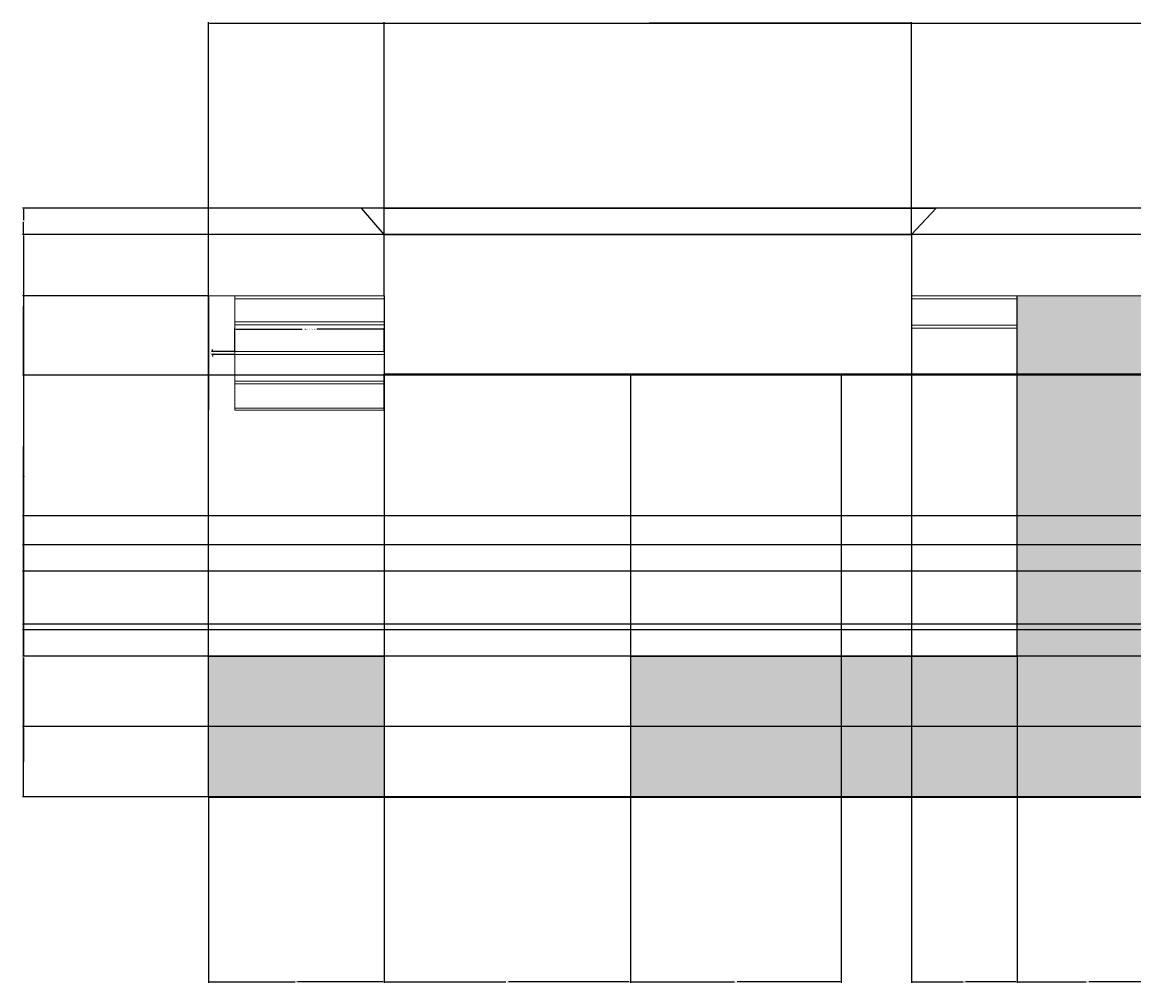
# Model space of a CAD drawing. Units: inches. Extents: x 2121 to 2815, y 1818 to 2233.
# Tile 1 of 6: x 2121 to 2311, y 1818 to 1982. Entities that reach past the tile are written whole.
import ezdxf

# ---------------------------------------------------------------- set-up
doc = ezdxf.new("R2010")
doc.units = ezdxf.units.IN
for name, color, linetype, lineweight in [('A-ANNO-DIMS', 2, 'Continuous', 18), ('A-ELEV', 7, 'Continuous', 25), ('A-ELEV-GRDE', 7, 'Continuous', 35), ('A-ELEV-SLAT', 7, 'Continuous', 18), ('A-WALL-COPG', 7, 'Continuous', 25), ('A-WALL-PATT', 8, 'Continuous', 13)]:
    doc.layers.add(name, color=color, linetype=linetype, lineweight=lineweight)
doc.styles.get("Standard").update_dxf_attribs({"font": 'arial.ttf'})
doc.dimstyles.get("Standard").update_dxf_attribs({"dimtxt": 0.18, "dimasz": 0.18, "dimexe": 0.18, "dimexo": 0.0625, "dimgap": 0.09, "dimtad": 0, "dimtih": 1, "dimtoh": 1, "dimdec": 4, "dimzin": 0, "dimdsep": 46, "dimtxsty": 'Standard', "dimcen": 0.09, "dimadec": 0, "dimazin": 0, "dimtfac": 1, "dimtdec": 4, "dimtofl": 0, "dimtmove": 0, "dimatfit": 3, "dimfxl": 1, "dimtolj": 1, "dimtzin": 0, "dimarcsym": 0})

# ---------------------------------------------------------------- blocks, each defined once
blk = doc.blocks.new('WALL-SLAT-25_5')
for p, q in [((0, 0.5), (25.5, 0.5)), ((0, 0), (25.5, 0))]:
    blk.add_line(p, q)
blk = doc.blocks.new('*D8')
at = {"layer": 'A-ANNO-DIMS', "color": 0, "lineweight": -2, "transparency": 16777216}
for p, q in [((2157.33, 1925.97), (2157.33, 1929.92)), ((2157.51, 1929.74), (2168.82, 1929.74)), ((2182.65, 1929.74), (2171.35, 1929.74)), ((2182.83, 1925.97), (2182.83, 1929.92))]:
    blk.add_line(p, q, dxfattribs=at)
at = {"layer": 'A-ANNO-DIMS', "color": 0, "transparency": 16777216}
for points in [[(2157.51, 1929.77), (2157.51, 1929.71), (2157.33, 1929.74)], [(2182.65, 1929.77), (2182.65, 1929.71), (2182.83, 1929.74)]]:
    blk.add_solid(points, dxfattribs=at)
at = {"layer": 'Defpoints', "color": 0, "transparency": 16777216}
for p in [(2182.83, 1929.74), (2157.33, 1925.91), (2182.83, 1925.91)]:
    blk.add_point(p, dxfattribs=at)
at = {"layer": 'A-ANNO-DIMS', "color": 0, "transparency": 16777216, "insert": (2170.08, 1929.74), "char_height": 0.18, "attachment_point": 5}
blk.add_mtext('\\A1;LONG SLAT 26 TYP.', dxfattribs=at)
blk = doc.blocks.new('*D9')
at = {"layer": 'A-ANNO-DIMS', "color": 0, "lineweight": -2, "transparency": 16777216}
for p, q in [((2157.27, 1925.91), (2153.33, 1925.91)), ((2157.27, 1925.41), (2153.33, 1925.41)), ((2153.51, 1926.09), (2153.51, 1926.27)), ((2153.51, 1925.23), (2153.51, 1925.05))]:
    blk.add_line(p, q, dxfattribs=at)
at = {"layer": 'A-ANNO-DIMS', "color": 0, "transparency": 16777216}
for points in [[(2153.48, 1926.09), (2153.54, 1926.09), (2153.51, 1925.91)], [(2153.48, 1925.23), (2153.54, 1925.23), (2153.51, 1925.41)]]:
    blk.add_solid(points, dxfattribs=at)
at = {"layer": 'Defpoints', "color": 0, "transparency": 16777216}
for p in [(2153.51, 1925.91), (2157.33, 1925.91), (2157.33, 1925.41)]:
    blk.add_point(p, dxfattribs=at)
at = {"layer": 'A-ANNO-DIMS', "color": 0, "transparency": 16777216, "insert": (2153.51, 1925.66), "char_height": 0.18, "attachment_point": 5}
blk.add_mtext('\\A1;1 TYP.', dxfattribs=at)
blk = doc.blocks.new('*D43')
at = {"layer": 'A-ANNO-DIMS', "color": 0, "lineweight": -2, "transparency": 16777216}
for p, q in [((2152.83, 1935.47), (2152.83, 1982.13)), ((2153.01, 1981.95), (2398.33, 1981.95)), ((2644.45, 1981.95), (2399.13, 1981.95)), ((2644.63, 1950.47), (2644.63, 1982.13))]:
    blk.add_line(p, q, dxfattribs=at)
at = {"layer": 'A-ANNO-DIMS', "color": 0, "transparency": 16777216}
for points in [[(2153.01, 1981.98), (2153.01, 1981.92), (2152.83, 1981.95)], [(2644.45, 1981.98), (2644.45, 1981.92), (2644.63, 1981.95)]]:
    blk.add_solid(points, dxfattribs=at)
at = {"layer": 'Defpoints', "color": 0, "transparency": 16777216}
for p in [(2644.63, 1981.95), (2644.63, 1950.41), (2152.83, 1935.41)]:
    blk.add_point(p, dxfattribs=at)
at = {"layer": 'A-ANNO-DIMS', "color": 0, "transparency": 16777216, "insert": (2398.73, 1981.95), "char_height": 0.18, "attachment_point": 5}
blk.add_mtext('\\A1;491.8', dxfattribs=at)
blk = doc.blocks.new('*D45')
at = {"layer": 'A-ANNO-DIMS', "color": 0, "lineweight": -2, "transparency": 16777216}
for p, q in [((2152.77, 1873.91), (2121.11, 1873.91)), ((2121.29, 1873.73), (2121.29, 1862.09)), ((2121.29, 1850.09), (2121.29, 1861.73)), ((2152.77, 1849.91), (2121.11, 1849.91))]:
    blk.add_line(p, q, dxfattribs=at)
at = {"layer": 'A-ANNO-DIMS', "color": 0, "transparency": 16777216}
for points in [[(2121.26, 1873.73), (2121.32, 1873.73), (2121.29, 1873.91)], [(2121.26, 1850.09), (2121.32, 1850.09), (2121.29, 1849.91)]]:
    blk.add_solid(points, dxfattribs=at)
at = {"layer": 'Defpoints', "color": 0, "transparency": 16777216}
for p in [(2121.29, 1873.91), (2152.83, 1873.91), (2152.83, 1849.91)]:
    blk.add_point(p, dxfattribs=at)
at = {"layer": 'A-ANNO-DIMS', "color": 0, "transparency": 16777216, "insert": (2121.29, 1861.91), "char_height": 0.18, "attachment_point": 5}
blk.add_mtext('\\A1;24', dxfattribs=at)
blk = doc.blocks.new('*D46')
at = {"layer": 'A-ANNO-DIMS', "color": 0, "lineweight": -2, "transparency": 16777216}
for p, q in [((2152.77, 1935.41), (2121.11, 1935.41)), ((2121.29, 1935.23), (2121.29, 1904.84)), ((2121.29, 1874.09), (2121.29, 1904.48)), ((2152.77, 1873.91), (2121.11, 1873.91))]:
    blk.add_line(p, q, dxfattribs=at)
at = {"layer": 'A-ANNO-DIMS', "color": 0, "transparency": 16777216}
for points in [[(2121.26, 1935.23), (2121.32, 1935.23), (2121.29, 1935.41)], [(2121.26, 1874.09), (2121.32, 1874.09), (2121.29, 1873.91)]]:
    blk.add_solid(points, dxfattribs=at)
at = {"layer": 'Defpoints', "color": 0, "transparency": 16777216}
for p in [(2121.29, 1935.41), (2152.83, 1935.41), (2152.83, 1873.91)]:
    blk.add_point(p, dxfattribs=at)
at = {"layer": 'A-ANNO-DIMS', "color": 0, "transparency": 16777216, "insert": (2121.29, 1904.66), "char_height": 0.18, "attachment_point": 5}
blk.add_mtext('\\A1;61.5', dxfattribs=at)
blk = doc.blocks.new('*D47')
at = {"layer": 'A-ANNO-DIMS', "color": 0, "lineweight": -2, "transparency": 16777216}
for p, q in [((2152.83, 1849.84), (2152.83, 1818.19)), ((2182.83, 1849.84), (2182.83, 1818.19)), ((2153.01, 1818.37), (2167.61, 1818.37)), ((2182.65, 1818.37), (2168.05, 1818.37))]:
    blk.add_line(p, q, dxfattribs=at)
at = {"layer": 'A-ANNO-DIMS', "color": 0, "transparency": 16777216}
for points in [[(2153.01, 1818.4), (2153.01, 1818.34), (2152.83, 1818.37)], [(2182.65, 1818.4), (2182.65, 1818.34), (2182.83, 1818.37)]]:
    blk.add_solid(points, dxfattribs=at)
at = {"layer": 'Defpoints', "color": 0, "transparency": 16777216}
for p in [(2152.83, 1849.91), (2182.83, 1849.91), (2182.83, 1818.37)]:
    blk.add_point(p, dxfattribs=at)
at = {"layer": 'A-ANNO-DIMS', "color": 0, "transparency": 16777216, "insert": (2167.83, 1818.37), "char_height": 0.18, "attachment_point": 5}
blk.add_mtext('\\A1;30', dxfattribs=at)
blk = doc.blocks.new('*D48')
at = {"layer": 'A-ANNO-DIMS', "color": 0, "lineweight": -2, "transparency": 16777216}
for p, q in [((2182.83, 1849.84), (2182.83, 1818.19)), ((2224.83, 1849.84), (2224.83, 1818.19)), ((2183.01, 1818.37), (2203.61, 1818.37)), ((2224.65, 1818.37), (2204.05, 1818.37))]:
    blk.add_line(p, q, dxfattribs=at)
at = {"layer": 'A-ANNO-DIMS', "color": 0, "transparency": 16777216}
for points in [[(2183.01, 1818.4), (2183.01, 1818.34), (2182.83, 1818.37)], [(2224.65, 1818.4), (2224.65, 1818.34), (2224.83, 1818.37)]]:
    blk.add_solid(points, dxfattribs=at)
at = {"layer": 'Defpoints', "color": 0, "transparency": 16777216}
for p in [(2182.83, 1849.91), (2224.83, 1849.91), (2224.83, 1818.37)]:
    blk.add_point(p, dxfattribs=at)
at = {"layer": 'A-ANNO-DIMS', "color": 0, "transparency": 16777216, "insert": (2203.83, 1818.37), "char_height": 0.18, "attachment_point": 5}
blk.add_mtext('\\A1;42', dxfattribs=at)
blk = doc.blocks.new('*D49')
at = {"layer": 'A-ANNO-DIMS', "color": 0, "lineweight": -2, "transparency": 16777216}
for p, q in [((2182.83, 1945.97), (2182.83, 1982.13)), ((2183.01, 1981.95), (2227.61, 1981.95)), ((2272.65, 1981.95), (2228.05, 1981.95)), ((2272.83, 1945.97), (2272.83, 1982.13))]:
    blk.add_line(p, q, dxfattribs=at)
at = {"layer": 'A-ANNO-DIMS', "color": 0, "transparency": 16777216}
for points in [[(2183.01, 1981.98), (2183.01, 1981.92), (2182.83, 1981.95)], [(2272.65, 1981.98), (2272.65, 1981.92), (2272.83, 1981.95)]]:
    blk.add_solid(points, dxfattribs=at)
at = {"layer": 'Defpoints', "color": 0, "transparency": 16777216}
for p in [(2272.83, 1981.95), (2182.83, 1945.91), (2272.83, 1945.91)]:
    blk.add_point(p, dxfattribs=at)
at = {"layer": 'A-ANNO-DIMS', "color": 0, "transparency": 16777216, "insert": (2227.83, 1981.95), "char_height": 0.18, "attachment_point": 5}
blk.add_mtext('\\A1;90', dxfattribs=at)
blk = doc.blocks.new('*D50')
at = {"layer": 'A-ANNO-DIMS', "color": 0, "lineweight": -2, "transparency": 16777216}
for p, q in [((2272.83, 1873.84), (2272.83, 1818.19)), ((2290.83, 1873.84), (2290.83, 1818.19)), ((2273.01, 1818.37), (2281.62, 1818.37)), ((2290.65, 1818.37), (2282.04, 1818.37))]:
    blk.add_line(p, q, dxfattribs=at)
at = {"layer": 'A-ANNO-DIMS', "color": 0, "transparency": 16777216}
for points in [[(2273.01, 1818.4), (2273.01, 1818.34), (2272.83, 1818.37)], [(2290.65, 1818.4), (2290.65, 1818.34), (2290.83, 1818.37)]]:
    blk.add_solid(points, dxfattribs=at)
at = {"layer": 'Defpoints', "color": 0, "transparency": 16777216}
for p in [(2272.83, 1873.91), (2290.83, 1873.91), (2290.83, 1818.37)]:
    blk.add_point(p, dxfattribs=at)
at = {"layer": 'A-ANNO-DIMS', "color": 0, "transparency": 16777216, "insert": (2281.83, 1818.37), "char_height": 0.18, "attachment_point": 5}
blk.add_mtext('\\A1;18', dxfattribs=at)
blk = doc.blocks.new('*D51')
at = {"layer": 'A-ANNO-DIMS', "color": 0, "lineweight": -2, "transparency": 16777216}
for p, q in [((2290.83, 1873.84), (2290.83, 1818.19)), ((2314.83, 1873.84), (2314.83, 1818.19)), ((2291.01, 1818.37), (2302.61, 1818.37)), ((2314.65, 1818.37), (2303.05, 1818.37))]:
    blk.add_line(p, q, dxfattribs=at)
at = {"layer": 'A-ANNO-DIMS', "color": 0, "transparency": 16777216}
for points in [[(2291.01, 1818.4), (2291.01, 1818.34), (2290.83, 1818.37)], [(2314.65, 1818.4), (2314.65, 1818.34), (2314.83, 1818.37)]]:
    blk.add_solid(points, dxfattribs=at)
at = {"layer": 'Defpoints', "color": 0, "transparency": 16777216}
for p in [(2290.83, 1873.91), (2314.83, 1873.91), (2314.83, 1818.37)]:
    blk.add_point(p, dxfattribs=at)
at = {"layer": 'A-ANNO-DIMS', "color": 0, "transparency": 16777216, "insert": (2302.83, 1818.37), "char_height": 0.18, "attachment_point": 5}
blk.add_mtext('\\A1;24', dxfattribs=at)
blk = doc.blocks.new('*D59')
at = {"layer": 'A-ANNO-DIMS', "color": 0, "lineweight": -2, "transparency": 16777216}
for p, q in [((2182.9, 1922.1), (2815, 1922.1)), ((2814.82, 1921.92), (2814.82, 1886.18)), ((2814.82, 1850.09), (2814.82, 1885.82)), ((2182.9, 1849.91), (2815, 1849.91))]:
    blk.add_line(p, q, dxfattribs=at)
at = {"layer": 'A-ANNO-DIMS', "color": 0, "transparency": 16777216}
for points in [[(2814.79, 1921.92), (2814.85, 1921.92), (2814.82, 1922.1)], [(2814.79, 1850.09), (2814.85, 1850.09), (2814.82, 1849.91)]]:
    blk.add_solid(points, dxfattribs=at)
at = {"layer": 'Defpoints', "color": 0, "transparency": 16777216}
for p in [(2182.83, 1922.1), (2814.82, 1922.1), (2182.83, 1849.91)]:
    blk.add_point(p, dxfattribs=at)
at = {"layer": 'A-ANNO-DIMS', "color": 0, "transparency": 16777216, "insert": (2814.82, 1886), "char_height": 0.18, "attachment_point": 5}
blk.add_mtext('\\A1;72.2', dxfattribs=at)
blk = doc.blocks.new('*D60')
at = {"layer": 'A-ANNO-DIMS', "color": 0, "lineweight": -2, "transparency": 16777216}
for p, q in [((2224.83, 1873.84), (2224.83, 1818.19)), ((2260.83, 1873.84), (2260.83, 1818.19)), ((2225.01, 1818.37), (2242.61, 1818.37)), ((2260.65, 1818.37), (2243.05, 1818.37))]:
    blk.add_line(p, q, dxfattribs=at)
at = {"layer": 'A-ANNO-DIMS', "color": 0, "transparency": 16777216}
for points in [[(2225.01, 1818.4), (2225.01, 1818.34), (2224.83, 1818.37)], [(2260.65, 1818.4), (2260.65, 1818.34), (2260.83, 1818.37)]]:
    blk.add_solid(points, dxfattribs=at)
at = {"layer": 'Defpoints', "color": 0, "transparency": 16777216}
for p in [(2224.83, 1873.91), (2260.83, 1873.91), (2260.83, 1818.37)]:
    blk.add_point(p, dxfattribs=at)
at = {"layer": 'A-ANNO-DIMS', "color": 0, "transparency": 16777216, "insert": (2242.83, 1818.37), "char_height": 0.18, "attachment_point": 5}
blk.add_mtext('\\A1;36', dxfattribs=at)
blk = doc.blocks.new('*D61')
at = {"layer": 'A-ANNO-DIMS', "color": 0, "lineweight": -2, "transparency": 16777216}
for p, q in [((2314.77, 1861.91), (2121.11, 1861.91)), ((2121.29, 1861.73), (2121.29, 1856.09)), ((2121.29, 1850.09), (2121.29, 1855.73)), ((2314.77, 1849.91), (2121.11, 1849.91))]:
    blk.add_line(p, q, dxfattribs=at)
at = {"layer": 'A-ANNO-DIMS', "color": 0, "transparency": 16777216}
for points in [[(2121.26, 1861.73), (2121.32, 1861.73), (2121.29, 1861.91)], [(2121.26, 1850.09), (2121.32, 1850.09), (2121.29, 1849.91)]]:
    blk.add_solid(points, dxfattribs=at)
at = {"layer": 'Defpoints', "color": 0, "transparency": 16777216}
for p in [(2121.29, 1861.91), (2314.83, 1861.91), (2314.83, 1849.91)]:
    blk.add_point(p, dxfattribs=at)
at = {"layer": 'A-ANNO-DIMS', "color": 0, "transparency": 16777216, "insert": (2121.29, 1855.91), "char_height": 0.18, "attachment_point": 5}
blk.add_mtext('\\A1;12', dxfattribs=at)
blk = doc.blocks.new('*D63')
at = {"layer": 'A-ANNO-DIMS', "color": 0, "lineweight": -2, "transparency": 16777216}
for p, q in [((2347.77, 1892.91), (2121.11, 1892.91)), ((2121.29, 1892.73), (2121.29, 1890.84)), ((2121.29, 1888.59), (2121.29, 1890.48)), ((2347.77, 1888.41), (2121.11, 1888.41))]:
    blk.add_line(p, q, dxfattribs=at)
at = {"layer": 'A-ANNO-DIMS', "color": 0, "transparency": 16777216}
for points in [[(2121.26, 1892.73), (2121.32, 1892.73), (2121.29, 1892.91)], [(2121.26, 1888.59), (2121.32, 1888.59), (2121.29, 1888.41)]]:
    blk.add_solid(points, dxfattribs=at)
at = {"layer": 'Defpoints', "color": 0, "transparency": 16777216}
for p in [(2121.29, 1892.91), (2347.83, 1892.91), (2347.83, 1888.41)]:
    blk.add_point(p, dxfattribs=at)
at = {"layer": 'A-ANNO-DIMS', "color": 0, "transparency": 16777216, "insert": (2121.29, 1890.66), "char_height": 0.18, "attachment_point": 5}
blk.add_mtext('\\A1;4.5', dxfattribs=at)
blk = doc.blocks.new('*D64')
at = {"layer": 'A-ANNO-DIMS', "color": 0, "lineweight": -2, "transparency": 16777216}
for p, q in [((2347.77, 1879.41), (2121.11, 1879.41)), ((2121.29, 1879.23), (2121.29, 1876.84)), ((2121.29, 1874.09), (2121.29, 1876.48)), ((2314.77, 1873.91), (2121.11, 1873.91))]:
    blk.add_line(p, q, dxfattribs=at)
at = {"layer": 'A-ANNO-DIMS', "color": 0, "transparency": 16777216}
for points in [[(2121.26, 1879.23), (2121.32, 1879.23), (2121.29, 1879.41)], [(2121.26, 1874.09), (2121.32, 1874.09), (2121.29, 1873.91)]]:
    blk.add_solid(points, dxfattribs=at)
at = {"layer": 'Defpoints', "color": 0, "transparency": 16777216}
for p in [(2121.29, 1879.41), (2347.83, 1879.41), (2314.83, 1873.91)]:
    blk.add_point(p, dxfattribs=at)
at = {"layer": 'A-ANNO-DIMS', "color": 0, "transparency": 16777216, "insert": (2121.29, 1876.66), "char_height": 0.18, "attachment_point": 5}
blk.add_mtext('\\A1;5.5', dxfattribs=at)
blk = doc.blocks.new('*D65')
at = {"layer": 'A-ANNO-DIMS', "color": 0, "lineweight": -2, "transparency": 16777216}
for p, q in [((2619.77, 1897.91), (2121.11, 1897.91)), ((2121.29, 1897.73), (2121.29, 1874.09)), ((2121.29, 1850.09), (2121.29, 1873.73)), ((2619.77, 1849.91), (2121.11, 1849.91))]:
    blk.add_line(p, q, dxfattribs=at)
at = {"layer": 'A-ANNO-DIMS', "color": 0, "transparency": 16777216}
for points in [[(2121.26, 1897.73), (2121.32, 1897.73), (2121.29, 1897.91)], [(2121.26, 1850.09), (2121.32, 1850.09), (2121.29, 1849.91)]]:
    blk.add_solid(points, dxfattribs=at)
at = {"layer": 'Defpoints', "color": 0, "transparency": 16777216}
for p in [(2121.29, 1897.91), (2619.83, 1897.91), (2619.83, 1849.91)]:
    blk.add_point(p, dxfattribs=at)
at = {"layer": 'A-ANNO-DIMS', "color": 0, "transparency": 16777216, "insert": (2121.29, 1873.91), "char_height": 0.18, "attachment_point": 5}
blk.add_mtext('\\A1;48', dxfattribs=at)
blk = doc.blocks.new('*D66')
at = {"layer": 'A-ANNO-DIMS', "color": 0, "lineweight": -2, "transparency": 16777216}
for p, q in [((2619.77, 1921.91), (2121.11, 1921.91)), ((2121.29, 1921.73), (2121.29, 1910.09)), ((2121.29, 1898.09), (2121.29, 1909.73)), ((2619.77, 1897.91), (2121.11, 1897.91))]:
    blk.add_line(p, q, dxfattribs=at)
at = {"layer": 'A-ANNO-DIMS', "color": 0, "transparency": 16777216}
for points in [[(2121.26, 1921.73), (2121.32, 1921.73), (2121.29, 1921.91)], [(2121.26, 1898.09), (2121.32, 1898.09), (2121.29, 1897.91)]]:
    blk.add_solid(points, dxfattribs=at)
at = {"layer": 'Defpoints', "color": 0, "transparency": 16777216}
for p in [(2121.29, 1921.91), (2619.83, 1921.91), (2619.83, 1897.91)]:
    blk.add_point(p, dxfattribs=at)
at = {"layer": 'A-ANNO-DIMS', "color": 0, "transparency": 16777216, "insert": (2121.29, 1909.91), "char_height": 0.18, "attachment_point": 5}
blk.add_mtext('\\A1;24', dxfattribs=at)
blk = doc.blocks.new('*D72')
at = {"layer": 'A-ANNO-DIMS', "color": 0, "lineweight": -2, "transparency": 16777216}
for p, q in [((2760.77, 1861.91), (2121.11, 1861.91)), ((2121.29, 1861.73), (2121.29, 1856.09)), ((2121.29, 1850.09), (2121.29, 1855.73)), ((2760.77, 1849.91), (2121.11, 1849.91))]:
    blk.add_line(p, q, dxfattribs=at)
at = {"layer": 'A-ANNO-DIMS', "color": 0, "transparency": 16777216}
for points in [[(2121.26, 1861.73), (2121.32, 1861.73), (2121.29, 1861.91)], [(2121.26, 1850.09), (2121.32, 1850.09), (2121.29, 1849.91)]]:
    blk.add_solid(points, dxfattribs=at)
at = {"layer": 'Defpoints', "color": 0, "transparency": 16777216}
for p in [(2121.29, 1861.91), (2760.83, 1861.91), (2760.83, 1849.91)]:
    blk.add_point(p, dxfattribs=at)
at = {"layer": 'A-ANNO-DIMS', "color": 0, "transparency": 16777216, "insert": (2121.29, 1855.91), "char_height": 0.18, "attachment_point": 5}
blk.add_mtext('\\A1;12', dxfattribs=at)
blk = doc.blocks.new('*D73')
at = {"layer": 'A-ANNO-DIMS', "color": 0, "lineweight": -2, "transparency": 16777216}
for p, q in [((2765.27, 1873.91), (2121.11, 1873.91)), ((2121.29, 1873.73), (2121.29, 1868.09)), ((2121.29, 1862.09), (2121.29, 1867.73)), ((2760.77, 1861.91), (2121.11, 1861.91))]:
    blk.add_line(p, q, dxfattribs=at)
at = {"layer": 'A-ANNO-DIMS', "color": 0, "transparency": 16777216}
for points in [[(2121.26, 1873.73), (2121.32, 1873.73), (2121.29, 1873.91)], [(2121.26, 1862.09), (2121.32, 1862.09), (2121.29, 1861.91)]]:
    blk.add_solid(points, dxfattribs=at)
at = {"layer": 'Defpoints', "color": 0, "transparency": 16777216}
for p in [(2121.29, 1873.91), (2765.33, 1873.91), (2760.83, 1861.91)]:
    blk.add_point(p, dxfattribs=at)
at = {"layer": 'A-ANNO-DIMS', "color": 0, "transparency": 16777216, "insert": (2121.29, 1867.91), "char_height": 0.18, "attachment_point": 5}
blk.add_mtext('\\A1;12', dxfattribs=at)
blk = doc.blocks.new('*D74')
at = {"layer": 'A-ANNO-DIMS', "color": 0, "lineweight": -2, "transparency": 16777216}
for p, q in [((2765.27, 1921.91), (2121.11, 1921.91)), ((2121.29, 1921.73), (2121.29, 1898.09)), ((2121.29, 1874.09), (2121.29, 1897.73)), ((2765.27, 1873.91), (2121.11, 1873.91))]:
    blk.add_line(p, q, dxfattribs=at)
at = {"layer": 'A-ANNO-DIMS', "color": 0, "transparency": 16777216}
for points in [[(2121.26, 1921.73), (2121.32, 1921.73), (2121.29, 1921.91)], [(2121.26, 1874.09), (2121.32, 1874.09), (2121.29, 1873.91)]]:
    blk.add_solid(points, dxfattribs=at)
at = {"layer": 'Defpoints', "color": 0, "transparency": 16777216}
for p in [(2121.29, 1921.91), (2765.33, 1921.91), (2765.33, 1873.91)]:
    blk.add_point(p, dxfattribs=at)
at = {"layer": 'A-ANNO-DIMS', "color": 0, "transparency": 16777216, "insert": (2121.29, 1897.91), "char_height": 0.18, "attachment_point": 5}
blk.add_mtext('\\A1;48', dxfattribs=at)
blk = doc.blocks.new('*D75')
at = {"layer": 'A-ANNO-DIMS', "color": 0, "lineweight": -2, "transparency": 16777216}
for p, q in [((2760.77, 1945.91), (2121.11, 1945.91)), ((2121.29, 1945.73), (2121.29, 1934.09)), ((2121.29, 1922.09), (2121.29, 1933.73)), ((2760.77, 1921.91), (2121.11, 1921.91))]:
    blk.add_line(p, q, dxfattribs=at)
at = {"layer": 'A-ANNO-DIMS', "color": 0, "transparency": 16777216}
for points in [[(2121.26, 1945.73), (2121.32, 1945.73), (2121.29, 1945.91)], [(2121.26, 1922.09), (2121.32, 1922.09), (2121.29, 1921.91)]]:
    blk.add_solid(points, dxfattribs=at)
at = {"layer": 'Defpoints', "color": 0, "transparency": 16777216}
for p in [(2121.29, 1945.91), (2760.83, 1945.91), (2760.83, 1921.91)]:
    blk.add_point(p, dxfattribs=at)
at = {"layer": 'A-ANNO-DIMS', "color": 0, "transparency": 16777216, "insert": (2121.29, 1933.91), "char_height": 0.18, "attachment_point": 5}
blk.add_mtext('\\A1;24', dxfattribs=at)
blk = doc.blocks.new('*D76')
at = {"layer": 'A-ANNO-DIMS', "color": 0, "lineweight": -2, "transparency": 16777216}
for p, q in [((2756.87, 1950.41), (2121.11, 1950.41)), ((2121.29, 1950.23), (2121.29, 1948.34)), ((2121.29, 1946.09), (2121.29, 1947.98)), ((2760.77, 1945.91), (2121.11, 1945.91))]:
    blk.add_line(p, q, dxfattribs=at)
at = {"layer": 'A-ANNO-DIMS', "color": 0, "transparency": 16777216}
for points in [[(2121.26, 1950.23), (2121.32, 1950.23), (2121.29, 1950.41)], [(2121.26, 1946.09), (2121.32, 1946.09), (2121.29, 1945.91)]]:
    blk.add_solid(points, dxfattribs=at)
at = {"layer": 'Defpoints', "color": 0, "transparency": 16777216}
for p in [(2121.29, 1950.41), (2756.93, 1950.41), (2760.83, 1945.91)]:
    blk.add_point(p, dxfattribs=at)
at = {"layer": 'A-ANNO-DIMS', "color": 0, "transparency": 16777216, "insert": (2121.29, 1948.16), "char_height": 0.18, "attachment_point": 5}
blk.add_mtext('\\A1;4.5', dxfattribs=at)
blk = doc.blocks.new('*D82')
at = {"layer": 'A-ANNO-DIMS', "color": 0, "lineweight": -2, "transparency": 16777216}
for p, q in [((2769.77, 1878.41), (2121.11, 1878.41)), ((2121.29, 1878.23), (2121.29, 1876.34)), ((2121.29, 1874.09), (2121.29, 1875.98)), ((2769.77, 1873.91), (2121.11, 1873.91))]:
    blk.add_line(p, q, dxfattribs=at)
at = {"layer": 'A-ANNO-DIMS', "color": 0, "transparency": 16777216}
for points in [[(2121.26, 1878.23), (2121.32, 1878.23), (2121.29, 1878.41)], [(2121.26, 1874.09), (2121.32, 1874.09), (2121.29, 1873.91)]]:
    blk.add_solid(points, dxfattribs=at)
at = {"layer": 'Defpoints', "color": 0, "transparency": 16777216}
for p in [(2121.29, 1878.41), (2769.83, 1878.41), (2769.83, 1873.91)]:
    blk.add_point(p, dxfattribs=at)
at = {"layer": 'A-ANNO-DIMS', "color": 0, "transparency": 16777216, "insert": (2121.29, 1876.16), "char_height": 0.18, "attachment_point": 5}
blk.add_mtext('\\A1;4.5', dxfattribs=at)

msp = doc.modelspace()

# ---------------------------------------------------------------- hatches: boundary and pattern name
at = {"layer": 'A-WALL-PATT'}
h = msp.add_hatch(dxfattribs=at)
h.set_pattern_fill('DOTS', color=256)
h.paths.add_polyline_path([(2182.8326, 1873.9075), (2152.8326, 1873.9075), (2152.8326, 1849.9075), (2182.8326, 1849.9075)])
h.paths.add_polyline_path([(2404.8326, 1873.9075), (2314.8326, 1873.9075), (2314.8326, 1935.4075), (2290.8326, 1935.4075), (2290.8326, 1873.9075), (2272.8326, 1873.9075), (2224.8326, 1873.9075), (2224.8326, 1849.9075), (2314.8326, 1849.9075), (2314.8326, 1861.9075), (2404.8326, 1861.9075)])
h.paths.add_polyline_path([(2464.8326, 1934.9075), (2440.8326, 1934.9075), (2440.8326, 1873.9075), (2422.8326, 1873.9075), (2422.8326, 1849.9075), (2440.8326, 1849.9075), (2464.8326, 1849.9075), (2494.8326, 1849.9075), (2494.8326, 1873.9075), (2464.8326, 1873.9075)])

# ---------------------------------------------------------------- linework, layer by layer
at = {"layer": 'A-ELEV'}
for p, q in [((2182.8326, 1935.4075), (2182.8326, 1945.9075)), ((2272.8326, 1945.9075), (2272.8326, 1873.9075)), ((2152.8326, 1873.9075), (2152.8326, 1935.4075)), ((2152.8326, 1935.4075), (2152.8326, 1915.9075)), ((2182.8326, 1935.4075), (2182.8326, 1873.9075)), ((2290.8326, 1873.9075), (2290.8326, 1935.4075)), ((2182.8326, 1915.9075), (2182.8326, 1922.1005)), ((2182.8326, 1922.1005), (2272.8326, 1922.1005)), ((2224.8326, 1922.1005), (2224.8326, 1849.9075)), ((2260.8326, 1922.1005), (2260.8326, 1873.9075)), ((2152.8326, 1849.9075), (2152.8326, 1873.9075)), ((2152.8326, 1873.9075), (2182.8326, 1873.9075)), ((2182.8326, 1873.9075), (2182.8326, 1849.9075)), ((2224.8326, 1873.9075), (2290.8326, 1873.9075)), ((2272.8326, 1873.9075), (2290.8326, 1873.9075))]:
    msp.add_line(p, q, dxfattribs=at)
at = {"layer": 'A-ELEV-GRDE'}
msp.add_line((2152.8326, 1849.9075), (2778.8326, 1849.9075), dxfattribs=at)
at = {"layer": 'A-ELEV-SLAT'}
for p, q in [((2152.8326, 1935.4075), (2182.8326, 1935.4075)), ((2157.3326, 1935.4075), (2157.3326, 1915.9075)), ((2157.3326, 1934.9075), (2182.8326, 1934.9075)), ((2272.8326, 1935.4075), (2332.7939, 1935.4075)), ((2272.8326, 1934.9075), (2290.8326, 1934.9075)), ((2272.8326, 1930.4075), (2290.8326, 1930.4075)), ((2272.8326, 1929.9075), (2290.8326, 1929.9075)), ((2157.3326, 1920.8595), (2182.8326, 1920.8595)), ((2157.3326, 1920.4153), (2182.8326, 1920.4153)), ((2157.3326, 1916.2845), (2182.8326, 1916.2845)), ((2157.3326, 1915.9075), (2182.8326, 1915.9075))]:
    msp.add_line(p, q, dxfattribs=at)
at = {"layer": 'A-WALL-COPG'}
for p, q in [((2182.8326, 1950.4075), (2178.9596, 1950.4075)), ((2182.8326, 1945.9075), (2178.9596, 1950.4075)), ((2182.8326, 1950.4075), (2277.0124, 1950.4075)), ((2272.8326, 1945.9075), (2277.0124, 1950.4075)), ((2182.8326, 1945.9075), (2224.8326, 1945.9075)), ((2224.8326, 1945.9075), (2260.8326, 1945.9075)), ((2260.8326, 1945.9075), (2272.8326, 1945.9075))]:
    msp.add_line(p, q, dxfattribs=at)

# ---------------------------------------------------------------- block references
at = {"layer": 'A-ELEV-SLAT'}
for p in [(2157.3326, 1930.5068), (2157.3326, 1925.4121)]:
    msp.add_blockref('WALL-SLAT-25_5', p, dxfattribs=at)

# ---------------------------------------------------------------- dimensions: what is measured, and where the dimension line sits
at = {"layer": 'A-ANNO-DIMS'}
for base, p1, p2, override, picture, middle in [((2644.6318, 1981.9475), (2152.8326, 1935.4075), (2644.6318, 1950.4075), {"dimdec": 1, "dimlfac": 1, "dimrnd": 0, "dimzin": 0, "dimdsep": 46, "dimlunit": 2}, '*D43', (2398.7322, 1981.9475)), ((2272.8326, 1981.9475), (2182.8326, 1945.9075), (2272.8326, 1945.9075), {"dimdec": 0, "dimlfac": 1, "dimrnd": 0, "dimzin": 0, "dimdsep": 46, "dimlunit": 2}, '*D49', (2227.8326, 1981.9475)), ((2260.8326, 1818.3675), (2224.8326, 1873.9075), (2260.8326, 1873.9075), {"dimdec": 0, "dimlfac": 1, "dimrnd": 0, "dimzin": 0, "dimdsep": 46, "dimlunit": 2}, '*D60', (2242.8326, 1818.3675)), ((2290.8326, 1818.3675), (2272.8326, 1873.9075), (2290.8326, 1873.9075), {"dimdec": 0, "dimlfac": 1, "dimrnd": 0, "dimzin": 0, "dimdsep": 46, "dimlunit": 2}, '*D50', (2281.8326, 1818.3675)), ((2314.8326, 1818.3675), (2290.8326, 1873.9075), (2314.8326, 1873.9075), {"dimdec": 0, "dimlfac": 1, "dimrnd": 0, "dimzin": 0, "dimdsep": 46, "dimlunit": 2}, '*D51', (2302.8326, 1818.3675)), ((2182.8326, 1818.3675), (2152.8326, 1849.9075), (2182.8326, 1849.9075), {"dimdec": 0, "dimlfac": 1, "dimrnd": 0, "dimzin": 0, "dimdsep": 46, "dimlunit": 2}, '*D47', (2167.8326, 1818.3675)), ((2224.8326, 1818.3675), (2182.8326, 1849.9075), (2224.8326, 1849.9075), {"dimdec": 0, "dimlfac": 1, "dimrnd": 0, "dimzin": 0, "dimdsep": 46, "dimlunit": 2}, '*D48', (2203.8326, 1818.3675))]:
    dim = msp.add_linear_dim(base=base, p1=p1, p2=p2, dimstyle='Standard', override=override, dxfattribs=at)
    dim.commit()
    dim.dimension.update_dxf_attribs({"geometry": picture, "text_midpoint": middle})
for base, p1, p2, override, picture, middle in [((2121.2926, 1950.4075), (2760.8326, 1945.9075), (2756.9306, 1950.4075), {"dimdec": 1, "dimlfac": 1, "dimrnd": 0, "dimzin": 0, "dimdsep": 46, "dimlunit": 2}, '*D76', (2121.2926, 1948.1575)), ((2121.2926, 1945.9075), (2760.8326, 1921.9075), (2760.8326, 1945.9075), {"dimdec": 0, "dimlfac": 1, "dimrnd": 0, "dimzin": 0, "dimdsep": 46, "dimlunit": 2}, '*D75', (2121.2926, 1933.9075)), ((2121.2926, 1935.4075), (2152.8326, 1873.9075), (2152.8326, 1935.4075), {"dimdec": 1, "dimlfac": 1, "dimrnd": 0, "dimzin": 0, "dimdsep": 46, "dimlunit": 2}, '*D46', (2121.2926, 1904.6575)), ((2121.2926, 1921.9075), (2619.8326, 1897.9075), (2619.8326, 1921.9075), {"dimdec": 0, "dimlfac": 1, "dimrnd": 0, "dimzin": 0, "dimdsep": 46, "dimlunit": 2}, '*D66', (2121.2926, 1909.9075)), ((2121.2926, 1921.9075), (2765.3326, 1873.9075), (2765.3326, 1921.9075), {"dimdec": 0, "dimlfac": 1, "dimrnd": 0, "dimzin": 0, "dimdsep": 46, "dimlunit": 2}, '*D74', (2121.2926, 1897.9075)), ((2814.82, 1922.1005), (2182.8326, 1849.9075), (2182.8326, 1922.1005), {"dimdec": 1, "dimlfac": 1, "dimrnd": 0, "dimzin": 0, "dimdsep": 46, "dimlunit": 2}, '*D59', (2814.82, 1886.004)), ((2121.2926, 1897.9075), (2619.8326, 1849.9075), (2619.8326, 1897.9075), {"dimdec": 0, "dimlfac": 1, "dimrnd": 0, "dimzin": 0, "dimdsep": 46, "dimlunit": 2}, '*D65', (2121.2926, 1873.9075)), ((2121.2926, 1892.9075), (2347.8326, 1888.4075), (2347.8326, 1892.9075), {"dimdec": 1, "dimlfac": 1, "dimrnd": 0, "dimzin": 0, "dimdsep": 46, "dimlunit": 2}, '*D63', (2121.2926, 1890.6575)), ((2121.2926, 1879.4075), (2314.8326, 1873.9075), (2347.8326, 1879.4075), {"dimdec": 1, "dimlfac": 1, "dimrnd": 0, "dimzin": 0, "dimdsep": 46, "dimlunit": 2}, '*D64', (2121.2926, 1876.6575)), ((2121.2926, 1878.4075), (2769.8326, 1873.9075), (2769.8326, 1878.4075), {"dimdec": 1, "dimlfac": 1, "dimrnd": 0, "dimzin": 0, "dimdsep": 46, "dimlunit": 2}, '*D82', (2121.2926, 1876.1575)), ((2121.2926, 1873.9075), (2152.8326, 1849.9075), (2152.8326, 1873.9075), {"dimdec": 0, "dimlfac": 1, "dimrnd": 0, "dimzin": 0, "dimdsep": 46, "dimlunit": 2}, '*D45', (2121.2926, 1861.9075)), ((2121.2926, 1873.9075), (2760.8326, 1861.9075), (2765.3326, 1873.9075), {"dimdec": 0, "dimlfac": 1, "dimrnd": 0, "dimzin": 0, "dimdsep": 46, "dimlunit": 2}, '*D73', (2121.2926, 1867.9075)), ((2121.2926, 1861.9075), (2314.8326, 1849.9075), (2314.8326, 1861.9075), {"dimdec": 0, "dimlfac": 1, "dimrnd": 0, "dimzin": 0, "dimdsep": 46, "dimlunit": 2}, '*D61', (2121.2926, 1855.9075)), ((2121.2926, 1861.9075), (2760.8326, 1849.9075), (2760.8326, 1861.9075), {"dimdec": 0, "dimlfac": 1, "dimrnd": 0, "dimzin": 0, "dimdsep": 46, "dimlunit": 2}, '*D72', (2121.2926, 1855.9075))]:
    dim = msp.add_linear_dim(base=base, p1=p1, p2=p2, angle=90, dimstyle='Standard', override=override, dxfattribs=at)
    dim.commit()
    dim.dimension.update_dxf_attribs({"geometry": picture, "text_midpoint": middle})
dim = msp.add_linear_dim(base=(2182.8326405562, 1929.7370630836), p1=(2157.3326405562, 1925.9120630836), p2=(2182.8326405562, 1925.9120630836), text='LONG SLAT <> TYP.', dimstyle='Standard', override={"dimdec": 0, "dimlfac": 1, "dimrnd": 0, "dimzin": 0, "dimdsep": 46, "dimlunit": 2}, dxfattribs=at)
dim.commit()
dim.dimension.update_dxf_attribs({"geometry": '*D8', "text_midpoint": (2170.0826405562, 1929.7370630836)})
dim = msp.add_linear_dim(base=(2153.5076405562, 1925.9120630836), p1=(2157.3326405562, 1925.4120630836), p2=(2157.3326405562, 1925.9120630836), angle=90, text='<> TYP.', dimstyle='Standard', override={"dimdec": 0, "dimlfac": 1, "dimrnd": 0, "dimzin": 0, "dimdsep": 46, "dimlunit": 2}, dxfattribs=at)
dim.commit()
dim.dimension.update_dxf_attribs({"geometry": '*D9', "text_midpoint": (2153.5076405562, 1925.6620630836)})

doc.saveas('drawing.dxf')
